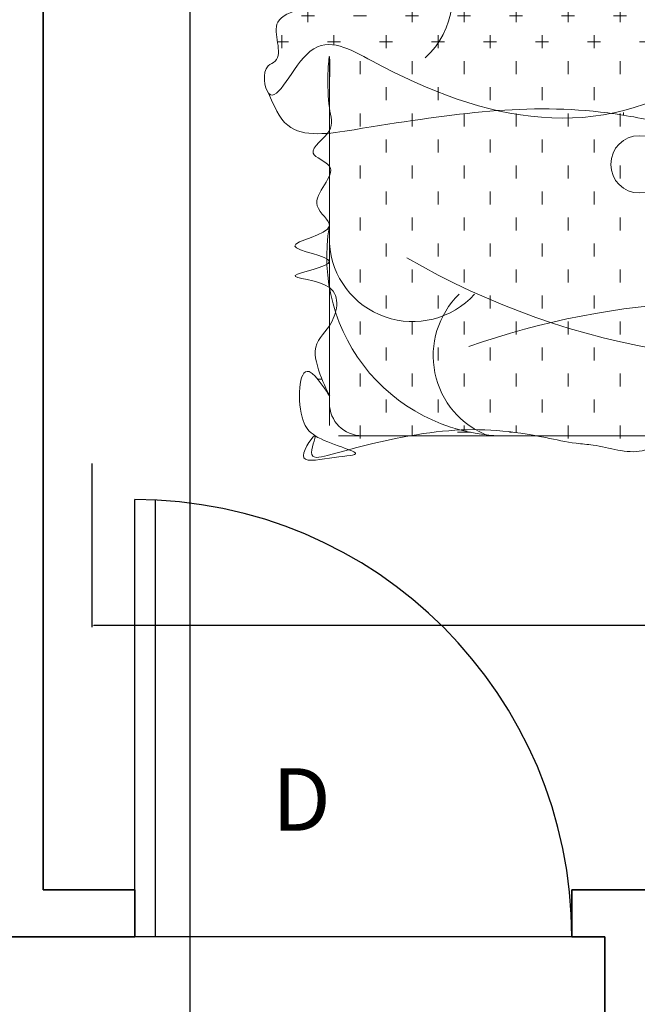
# Model space of a CAD drawing. Units: inches. Extents: x -26 to 575, y -18 to 513.
# Tile 11 of 28: x 136 to 196, y 324 to 418. Entities that reach past the tile are written whole.
import ezdxf

# ---------------------------------------------------------------- set-up
doc = ezdxf.new("R2010")
doc.units = ezdxf.units.IN
doc.header["$MEASUREMENT"] = 0
for name, color, linetype, lineweight in [('A-ANNO-DIMS', 2, 'Continuous', 18), ('A-ANNO-TEXT', 7, 'Continuous', 18), ('A-DOOR', 3, 'Continuous', 25), ('A-WALL', 7, 'Continuous', 35), ('Furniture', 8, 'Continuous', 15)]:
    doc.layers.add(name, color=color, linetype=linetype, lineweight=lineweight)
doc.styles.get("Standard").update_dxf_attribs({"font": 'arial.ttf', "height": 6})
doc.dimstyles.get("Standard").update_dxf_attribs({"dimtxt": 6, "dimasz": 0.18, "dimexe": 0.18, "dimexo": 0.0625, "dimgap": 0.09, "dimtad": 0, "dimtih": 1, "dimtoh": 1, "dimzin": 0, "dimdsep": 46, "dimlunit": 3, "dimtxsty": 'Standard', "dimcen": 0.09, "dimadec": 0, "dimazin": 0, "dimtfac": 1, "dimtofl": 0, "dimtmove": 0, "dimatfit": 3, "dimfxl": 1, "dimtolj": 1, "dimtzin": 0, "dimarcsym": 0})

# ---------------------------------------------------------------- blocks, each defined once
blk = doc.blocks.new('BED-DOUBLE-WITH-NIGHTSTANDS')
for p, q in [((1.925, 83.361), (1.925, 62.761)), ((82.669, 83.361), (82.669, 62.761)), ((21.61, 63.031), (21.61, 82.461)), ((22.828, 60.828), (22.828, 82.615)), ((81.883, 82.344), (81.883, 56.232)), ((102.354, 63.031), (102.354, 82.461)), ((10.269, 81.761), (8.938, 70.826)), ((23.226, 81.078), (0, 81.078)), ((21.24, 81.17), (81.883, 81.17)), ((103.97, 81.078), (80.744, 81.078)), ((20.889, 80.153), (2.667, 80.153)), ((2.667, 80.153), (2.667, 64.968)), ((20.889, 64.968), (20.889, 80.153)), ((82.669, 79.717), (21.062, 79.717)), ((101.633, 80.153), (83.411, 80.153)), ((83.411, 80.153), (83.411, 64.968)), ((101.633, 64.968), (101.633, 80.153)), ((92.567, 79.403), (92.567, 67.508)), ((14.667, 76.005), (4.51, 77.257)), ((25.057, 76.764), (22.828, 76.764)), ((41.168, 76.507), (40.96, 76.715)), ((41.168, 76.507), (41.434, 76.772)), ((41.169, 76.507), (41.169, 76.741)), ((56.226, 76.764), (41.357, 76.764)), ((43.997, 76.507), (43.732, 76.772)), ((43.997, 76.507), (43.997, 76.882)), ((43.997, 76.507), (44.262, 76.772)), ((46.825, 76.507), (46.56, 76.772)), ((46.825, 76.507), (47.09, 76.772)), ((46.826, 76.507), (46.826, 76.882)), ((57.003, 76.507), (56.737, 76.772)), ((57.003, 76.507), (57.003, 76.828)), ((57.003, 76.507), (57.268, 76.772)), ((81.883, 76.764), (59.394, 76.764)), ((59.831, 76.507), (59.594, 76.744)), ((59.831, 76.507), (59.831, 76.717)), ((59.831, 76.507), (60.018, 76.694)), ((8.056, 67.244), (12.026, 75.725)), ((12.026, 75.725), (14.235, 74.691)), ((11.458, 75.323), (8.122, 68.196)), ((11.769, 75.177), (11.458, 75.323)), ((25.612, 75.093), (25.347, 75.358)), ((25.612, 75.093), (25.612, 75.468)), ((25.612, 75.093), (25.877, 75.358)), ((28.44, 75.093), (28.175, 75.358)), ((28.44, 75.093), (28.706, 75.358)), ((28.441, 75.093), (28.441, 75.468)), ((31.269, 75.093), (31.004, 75.358)), ((31.269, 75.093), (31.269, 75.468)), ((31.269, 75.093), (31.534, 75.358)), ((34.097, 75.093), (33.832, 75.358)), ((34.097, 75.093), (34.362, 75.358)), ((34.098, 75.093), (34.098, 75.468)), ((36.926, 75.093), (36.661, 75.358)), ((36.926, 75.093), (36.926, 75.468)), ((36.926, 75.093), (37.191, 75.358)), ((39.754, 75.093), (39.489, 75.358)), ((39.754, 75.093), (40.019, 75.358)), ((39.755, 75.093), (39.755, 75.468)), ((42.583, 75.093), (42.317, 75.358)), ((42.583, 75.093), (42.583, 75.468)), ((42.583, 75.093), (42.848, 75.358)), ((45.411, 75.093), (45.146, 75.358)), ((45.411, 75.093), (45.411, 75.468)), ((45.411, 75.093), (45.676, 75.358)), ((48.239, 75.093), (47.974, 75.358)), ((48.239, 75.093), (48.505, 75.358)), ((48.24, 75.093), (48.24, 75.468)), ((51.068, 75.093), (50.803, 75.358)), ((51.068, 75.093), (51.068, 75.099)), ((51.068, 75.093), (51.07, 75.095)), ((53.004, 75.337), (53.025, 75.358)), ((55.588, 75.093), (55.323, 75.358)), ((55.588, 75.093), (55.854, 75.358)), ((55.589, 75.093), (55.589, 75.468)), ((58.417, 75.093), (58.152, 75.358)), ((58.417, 75.093), (58.417, 75.468)), ((58.417, 75.093), (58.682, 75.358)), ((61.245, 75.093), (60.98, 75.358)), ((61.245, 75.093), (61.51, 75.358)), ((61.246, 75.093), (61.246, 75.468)), ((64.074, 75.093), (63.809, 75.358)), ((64.074, 75.093), (64.074, 75.468)), ((64.074, 75.093), (64.339, 75.358)), ((66.902, 75.093), (66.637, 75.358)), ((66.902, 75.093), (67.167, 75.358)), ((66.903, 75.093), (66.903, 75.468)), ((69.731, 75.093), (69.465, 75.358)), ((69.731, 75.093), (69.731, 75.468)), ((69.731, 75.093), (69.996, 75.358)), ((72.559, 75.093), (72.294, 75.358)), ((72.559, 75.093), (72.559, 75.468)), ((72.559, 75.093), (72.824, 75.358)), ((75.387, 75.093), (75.122, 75.358)), ((75.387, 75.093), (75.653, 75.358)), ((75.388, 75.093), (75.388, 75.468)), ((78.216, 75.093), (77.951, 75.358)), ((78.216, 75.093), (78.216, 75.468)), ((78.216, 75.093), (78.481, 75.358)), ((14.235, 74.691), (10.265, 66.21)), ((19.14, 71.727), (13.978, 74.143)), ((27.026, 73.679), (26.761, 73.944)), ((27.026, 73.679), (27.291, 73.944)), ((27.027, 73.678), (27.027, 74.053)), ((29.855, 73.679), (29.589, 73.944)), ((29.855, 73.678), (29.855, 74.053)), ((29.855, 73.679), (30.12, 73.944)), ((32.683, 73.679), (32.418, 73.944)), ((32.683, 73.678), (32.683, 74.053)), ((32.683, 73.679), (32.948, 73.944)), ((35.512, 73.679), (35.246, 73.944)), ((35.512, 73.678), (35.512, 74.053)), ((35.512, 73.679), (35.777, 73.944)), ((38.34, 73.679), (38.075, 73.944)), ((38.34, 73.678), (38.34, 74.053)), ((38.34, 73.679), (38.605, 73.944)), ((41.168, 73.679), (40.903, 73.944)), ((41.168, 73.679), (41.434, 73.944)), ((41.169, 73.678), (41.169, 74.053)), ((43.997, 73.679), (43.732, 73.944)), ((43.997, 73.678), (43.997, 74.053)), ((43.997, 73.679), (44.262, 73.944)), ((46.825, 73.679), (46.56, 73.944)), ((46.825, 73.679), (47.09, 73.944)), ((46.826, 73.678), (46.826, 74.053)), ((49.654, 73.679), (49.388, 73.944)), ((49.654, 73.678), (49.654, 74.053)), ((49.654, 73.679), (49.919, 73.944)), ((54.174, 73.679), (53.909, 73.944)), ((54.174, 73.679), (54.439, 73.944)), ((54.175, 73.678), (54.175, 74.053)), ((57.003, 73.679), (56.737, 73.944)), ((57.003, 73.678), (57.003, 74.053)), ((57.003, 73.679), (57.268, 73.944)), ((59.831, 73.679), (59.566, 73.944)), ((59.831, 73.678), (59.831, 74.053)), ((59.831, 73.679), (60.096, 73.944)), ((62.66, 73.679), (62.394, 73.944)), ((62.66, 73.678), (62.66, 74.053)), ((62.66, 73.679), (62.925, 73.944)), ((65.488, 73.679), (65.223, 73.944)), ((65.488, 73.678), (65.488, 74.053)), ((65.488, 73.679), (65.753, 73.944)), ((68.316, 73.679), (68.051, 73.944)), ((68.316, 73.679), (68.582, 73.944)), ((68.317, 73.678), (68.317, 74.053)), ((71.145, 73.679), (70.88, 73.944)), ((71.145, 73.678), (71.145, 74.053)), ((71.145, 73.679), (71.41, 73.944)), ((73.973, 73.679), (73.708, 73.944)), ((73.973, 73.679), (74.238, 73.944)), ((73.974, 73.678), (73.974, 74.053)), ((76.802, 73.679), (76.536, 73.944)), ((76.802, 73.678), (76.802, 74.053)), ((76.802, 73.679), (77.067, 73.944)), ((79.63, 73.679), (79.365, 73.944)), ((79.63, 73.678), (79.63, 74.053)), ((79.63, 73.679), (79.895, 73.944)), ((13.242, 72.571), (11.033, 73.605)), ((14.129, 73), (11.598, 67.591)), ((17.984, 71.195), (14.129, 73)), ((98.466, 73.144), (86.668, 73.144)), ((25.612, 72.265), (25.347, 72.53)), ((25.612, 72.264), (25.612, 72.639)), ((25.612, 72.265), (25.877, 72.53)), ((28.44, 72.265), (28.175, 72.53)), ((28.44, 72.265), (28.706, 72.53)), ((28.441, 72.264), (28.441, 72.639)), ((31.269, 72.265), (31.004, 72.53)), ((31.269, 72.264), (31.269, 72.639)), ((31.269, 72.265), (31.534, 72.53)), ((34.097, 72.265), (33.832, 72.53)), ((34.097, 72.265), (34.362, 72.53)), ((34.098, 72.264), (34.098, 72.639)), ((36.926, 72.265), (36.661, 72.53)), ((36.926, 72.264), (36.926, 72.639)), ((36.926, 72.265), (37.191, 72.53)), ((39.754, 72.265), (39.489, 72.53)), ((39.754, 72.265), (40.019, 72.53)), ((39.755, 72.264), (39.755, 72.639)), ((42.583, 72.265), (42.317, 72.53)), ((42.583, 72.264), (42.583, 72.639)), ((42.583, 72.265), (42.848, 72.53)), ((45.411, 72.265), (45.146, 72.53)), ((45.411, 72.264), (45.411, 72.639)), ((45.411, 72.265), (45.676, 72.53)), ((48.239, 72.265), (47.974, 72.53)), ((48.239, 72.265), (48.505, 72.53)), ((48.24, 72.264), (48.24, 72.639)), ((55.588, 72.265), (55.323, 72.53)), ((55.588, 72.265), (55.854, 72.53)), ((55.589, 72.264), (55.589, 72.639)), ((58.417, 72.265), (58.152, 72.53)), ((58.417, 72.264), (58.417, 72.639)), ((58.417, 72.265), (58.682, 72.53)), ((61.245, 72.265), (60.98, 72.53)), ((61.245, 72.265), (61.51, 72.53)), ((61.246, 72.264), (61.246, 72.639)), ((64.074, 72.265), (63.809, 72.53)), ((64.074, 72.264), (64.074, 72.639)), ((64.074, 72.265), (64.339, 72.53)), ((66.902, 72.265), (66.637, 72.53)), ((66.902, 72.265), (67.167, 72.53)), ((66.903, 72.264), (66.903, 72.639)), ((69.731, 72.265), (69.465, 72.53)), ((69.731, 72.264), (69.731, 72.639)), ((69.731, 72.265), (69.996, 72.53)), ((72.559, 72.265), (72.294, 72.53)), ((72.559, 72.264), (72.559, 72.639)), ((72.559, 72.265), (72.824, 72.53)), ((75.387, 72.265), (75.122, 72.53)), ((75.387, 72.265), (75.653, 72.53)), ((75.388, 72.264), (75.388, 72.639)), ((78.216, 72.265), (77.951, 72.53)), ((78.216, 72.264), (78.216, 72.639)), ((78.216, 72.265), (78.481, 72.53)), ((15.452, 65.787), (17.984, 71.195)), ((15.804, 64.601), (19.14, 71.727)), ((24.198, 70.85), (23.972, 71.076)), ((24.198, 70.85), (24.198, 71.225)), ((24.198, 70.85), (24.463, 71.116)), ((27.026, 70.85), (26.761, 71.116)), ((27.026, 70.85), (27.291, 71.116)), ((27.027, 70.85), (27.027, 71.225)), ((29.855, 70.85), (29.589, 71.116)), ((29.855, 70.85), (29.855, 71.225)), ((29.855, 70.85), (30.12, 71.116)), ((32.683, 70.85), (32.418, 71.116)), ((32.683, 70.85), (32.683, 71.225)), ((32.683, 70.85), (32.948, 71.116)), ((35.512, 70.85), (35.246, 71.116)), ((35.512, 70.85), (35.512, 71.225)), ((35.512, 70.85), (35.777, 71.116)), ((38.34, 70.85), (38.075, 71.116)), ((38.34, 70.85), (38.34, 71.225)), ((38.34, 70.85), (38.605, 71.116)), ((41.168, 70.85), (40.903, 71.116)), ((41.168, 70.85), (41.434, 71.116)), ((41.169, 70.85), (41.169, 71.225)), ((43.997, 70.85), (43.732, 71.116)), ((43.997, 70.85), (43.997, 71.225)), ((43.997, 70.85), (44.262, 71.116)), ((46.825, 70.85), (46.56, 71.116)), ((46.825, 70.85), (47.09, 71.116)), ((46.826, 70.85), (46.826, 71.225)), ((49.654, 70.85), (49.388, 71.116)), ((49.654, 70.85), (49.654, 71.225)), ((49.654, 70.85), (49.919, 71.116)), ((54.174, 70.85), (53.909, 71.116)), ((54.174, 70.85), (54.439, 71.116)), ((54.175, 70.85), (54.175, 71.225)), ((57.003, 70.85), (56.737, 71.116)), ((57.003, 70.85), (57.003, 71.225)), ((57.003, 70.85), (57.268, 71.116)), ((59.831, 70.85), (59.566, 71.116)), ((59.831, 70.85), (59.831, 71.225)), ((59.831, 70.85), (60.096, 71.116)), ((62.66, 70.85), (62.394, 71.116)), ((62.66, 70.85), (62.66, 71.225)), ((62.66, 70.85), (62.925, 71.116)), ((65.488, 70.85), (65.223, 71.116)), ((65.488, 70.85), (65.488, 71.225)), ((65.488, 70.85), (65.753, 71.116)), ((68.316, 70.85), (68.051, 71.116)), ((68.316, 70.85), (68.582, 71.116)), ((68.317, 70.85), (68.317, 71.225)), ((71.145, 70.85), (70.88, 71.116)), ((71.145, 70.85), (71.145, 71.225)), ((71.145, 70.85), (71.41, 71.116)), ((73.973, 70.85), (73.708, 71.116)), ((73.973, 70.85), (74.238, 71.116)), ((73.974, 70.85), (73.974, 71.225)), ((76.802, 70.85), (76.536, 71.116)), ((76.802, 70.85), (76.802, 71.225)), ((76.802, 70.85), (77.067, 71.116)), ((79.63, 70.85), (79.365, 71.116)), ((79.63, 70.85), (79.63, 71.225)), ((79.63, 70.85), (79.895, 71.116)), ((11.136, 68.071), (8.927, 69.105)), ((25.612, 69.436), (25.347, 69.701)), ((25.612, 69.436), (25.612, 69.811)), ((25.612, 69.436), (25.877, 69.701)), ((28.44, 69.436), (28.175, 69.701)), ((28.44, 69.436), (28.706, 69.701)), ((28.441, 69.436), (28.441, 69.811)), ((31.269, 69.436), (31.004, 69.701)), ((31.269, 69.436), (31.269, 69.811)), ((31.269, 69.436), (31.534, 69.701)), ((34.097, 69.436), (33.832, 69.701)), ((34.097, 69.436), (34.362, 69.701)), ((34.098, 69.436), (34.098, 69.811)), ((36.926, 69.436), (36.661, 69.701)), ((36.926, 69.436), (36.926, 69.811)), ((36.926, 69.436), (37.191, 69.701)), ((39.754, 69.436), (39.489, 69.701)), ((39.754, 69.436), (40.019, 69.701)), ((39.755, 69.436), (39.755, 69.811)), ((42.583, 69.436), (42.317, 69.701)), ((42.583, 69.436), (42.583, 69.811)), ((42.583, 69.436), (42.848, 69.701)), ((45.411, 69.436), (45.146, 69.701)), ((45.411, 69.436), (45.411, 69.811)), ((45.411, 69.436), (45.676, 69.701)), ((48.239, 69.436), (47.974, 69.701)), ((48.239, 69.436), (48.505, 69.701)), ((48.24, 69.436), (48.24, 69.811)), ((51.052, 69.452), (50.803, 69.701)), ((53.007, 69.683), (53.025, 69.701)), ((55.588, 69.436), (55.323, 69.701)), ((55.588, 69.436), (55.854, 69.701)), ((55.589, 69.436), (55.589, 69.811)), ((58.417, 69.436), (58.152, 69.701)), ((58.417, 69.436), (58.417, 69.811)), ((58.417, 69.436), (58.682, 69.701)), ((61.245, 69.436), (60.98, 69.701)), ((61.245, 69.436), (61.51, 69.701)), ((61.246, 69.436), (61.246, 69.811)), ((64.074, 69.436), (63.809, 69.701)), ((64.074, 69.436), (64.074, 69.811)), ((64.074, 69.436), (64.339, 69.701)), ((66.902, 69.436), (66.637, 69.701)), ((66.902, 69.436), (67.167, 69.701)), ((66.903, 69.436), (66.903, 69.811)), ((69.731, 69.436), (69.465, 69.701)), ((69.731, 69.436), (69.731, 69.811)), ((69.731, 69.436), (69.996, 69.701)), ((72.559, 69.436), (72.294, 69.701)), ((72.559, 69.436), (72.559, 69.811)), ((72.559, 69.436), (72.824, 69.701)), ((75.387, 69.436), (75.122, 69.701)), ((75.387, 69.436), (75.653, 69.701)), ((75.388, 69.436), (75.388, 69.811)), ((78.216, 69.436), (77.951, 69.701)), ((78.216, 69.436), (78.216, 69.811)), ((78.216, 69.436), (78.481, 69.701)), ((8.122, 68.196), (8.434, 68.05)), ((24.198, 68.022), (23.933, 68.287)), ((24.198, 68.022), (24.198, 68.397)), ((24.198, 68.022), (24.463, 68.287)), ((27.026, 68.022), (26.761, 68.287)), ((27.026, 68.022), (27.291, 68.287)), ((27.027, 68.022), (27.027, 68.397)), ((29.855, 68.022), (29.589, 68.287)), ((29.855, 68.022), (29.855, 68.397)), ((29.855, 68.022), (30.12, 68.287)), ((32.683, 68.022), (32.418, 68.287)), ((32.683, 68.022), (32.683, 68.397)), ((32.683, 68.022), (32.948, 68.287)), ((35.512, 68.022), (35.246, 68.287)), ((35.512, 68.022), (35.512, 68.397)), ((35.512, 68.022), (35.777, 68.287)), ((38.34, 68.022), (38.075, 68.287)), ((38.34, 68.022), (38.34, 68.397)), ((38.34, 68.022), (38.605, 68.287)), ((41.168, 68.022), (40.903, 68.287)), ((41.168, 68.022), (41.434, 68.287)), ((41.169, 68.022), (41.169, 68.397)), ((43.997, 68.022), (43.732, 68.287)), ((43.997, 68.022), (43.997, 68.397)), ((43.997, 68.022), (44.262, 68.287)), ((46.825, 68.022), (46.56, 68.287)), ((46.825, 68.022), (47.09, 68.287)), ((46.826, 68.022), (46.826, 68.397)), ((49.654, 68.022), (49.388, 68.287)), ((49.654, 68.022), (49.654, 68.397)), ((49.654, 68.022), (49.919, 68.287)), ((54.174, 68.022), (53.909, 68.287)), ((54.174, 68.022), (54.439, 68.287)), ((54.175, 68.022), (54.175, 68.397)), ((57.003, 68.022), (56.737, 68.287)), ((57.003, 68.022), (57.003, 68.397)), ((57.003, 68.022), (57.268, 68.287)), ((59.831, 68.022), (59.566, 68.287)), ((59.831, 68.022), (59.831, 68.397)), ((59.831, 68.022), (60.096, 68.287)), ((62.66, 68.022), (62.394, 68.287)), ((62.66, 68.022), (62.66, 68.397)), ((62.66, 68.022), (62.925, 68.287)), ((65.488, 68.022), (65.223, 68.287)), ((65.488, 68.022), (65.488, 68.397)), ((65.488, 68.022), (65.753, 68.287)), ((68.316, 68.022), (68.051, 68.287)), ((68.316, 68.022), (68.582, 68.287)), ((68.317, 68.022), (68.317, 68.397)), ((71.145, 68.022), (70.88, 68.287)), ((71.145, 68.022), (71.145, 68.397)), ((71.145, 68.022), (71.41, 68.287)), ((73.973, 68.022), (73.708, 68.287)), ((73.973, 68.022), (74.238, 68.287)), ((73.974, 68.022), (73.974, 68.397)), ((76.802, 68.022), (76.536, 68.287)), ((76.802, 68.022), (76.802, 68.397)), ((76.802, 68.022), (77.067, 68.287)), ((79.63, 68.022), (79.365, 68.287)), ((79.63, 68.022), (79.63, 68.397)), ((79.63, 68.022), (79.895, 68.287)), ((10.265, 66.21), (8.056, 67.244)), ((11.598, 67.591), (15.452, 65.787)), ((10.642, 67.017), (15.804, 64.601)), ((25.612, 66.608), (25.347, 66.873)), ((25.612, 66.607), (25.612, 66.982)), ((25.612, 66.608), (25.877, 66.873)), ((28.44, 66.608), (28.175, 66.873)), ((28.44, 66.608), (28.706, 66.873)), ((28.441, 66.607), (28.441, 66.982)), ((31.269, 66.608), (31.004, 66.873)), ((31.269, 66.607), (31.269, 66.982)), ((31.269, 66.608), (31.534, 66.873)), ((34.097, 66.608), (33.832, 66.873)), ((34.097, 66.608), (34.362, 66.873)), ((34.098, 66.607), (34.098, 66.982)), ((36.926, 66.608), (36.661, 66.873)), ((36.926, 66.607), (36.926, 66.982)), ((36.926, 66.608), (37.191, 66.873)), ((39.754, 66.608), (39.489, 66.873)), ((39.754, 66.608), (40.019, 66.873)), ((39.755, 66.607), (39.755, 66.982)), ((42.583, 66.608), (42.317, 66.873)), ((42.583, 66.607), (42.583, 66.982)), ((42.583, 66.608), (42.848, 66.873)), ((45.411, 66.608), (45.146, 66.873)), ((45.411, 66.607), (45.411, 66.982)), ((45.411, 66.608), (45.676, 66.873)), ((48.239, 66.608), (47.974, 66.873)), ((48.239, 66.608), (48.505, 66.873)), ((48.24, 66.607), (48.24, 66.982)), ((51.068, 66.608), (50.803, 66.873)), ((51.068, 66.607), (51.068, 66.982)), ((51.068, 66.608), (51.333, 66.873)), ((52.76, 66.608), (52.495, 66.873)), ((52.76, 66.607), (52.76, 66.982)), ((52.76, 66.608), (53.025, 66.873)), ((55.588, 66.608), (55.323, 66.873)), ((55.588, 66.608), (55.854, 66.873)), ((55.589, 66.607), (55.589, 66.982)), ((58.417, 66.608), (58.152, 66.873)), ((58.417, 66.607), (58.417, 66.982)), ((58.417, 66.608), (58.682, 66.873)), ((61.245, 66.608), (60.98, 66.873)), ((61.245, 66.608), (61.51, 66.873)), ((61.246, 66.607), (61.246, 66.982)), ((64.074, 66.608), (63.809, 66.873)), ((64.074, 66.607), (64.074, 66.982)), ((64.074, 66.608), (64.339, 66.873)), ((66.902, 66.608), (66.637, 66.873)), ((66.902, 66.608), (67.167, 66.873)), ((66.903, 66.607), (66.903, 66.982)), ((69.731, 66.608), (69.465, 66.873)), ((69.731, 66.607), (69.731, 66.982)), ((69.731, 66.608), (69.996, 66.873)), ((72.559, 66.608), (72.294, 66.873)), ((72.559, 66.607), (72.559, 66.982)), ((72.559, 66.608), (72.824, 66.873)), ((75.387, 66.608), (75.122, 66.873)), ((75.387, 66.608), (75.653, 66.873)), ((75.388, 66.607), (75.388, 66.982)), ((78.216, 66.608), (77.951, 66.873)), ((78.216, 66.607), (78.216, 66.982)), ((78.216, 66.608), (78.481, 66.873)), ((81.044, 66.608), (80.779, 66.873)), ((81.044, 66.608), (81.253, 66.817)), ((81.045, 66.607), (81.045, 66.982)), ((24.198, 65.385), (24.198, 65.568)), ((24.295, 65.291), (24.463, 65.459)), ((27.026, 65.194), (26.761, 65.459)), ((27.026, 65.194), (27.291, 65.459)), ((27.027, 65.193), (27.027, 65.568)), ((29.855, 65.194), (29.589, 65.459)), ((29.855, 65.193), (29.855, 65.568)), ((29.855, 65.194), (30.12, 65.459)), ((32.683, 65.194), (32.418, 65.459)), ((32.683, 65.193), (32.683, 65.568)), ((32.683, 65.194), (32.948, 65.459)), ((35.335, 65.37), (35.246, 65.459)), ((35.512, 65.394), (35.512, 65.568)), ((35.743, 65.425), (35.777, 65.459)), ((46.774, 65.245), (46.56, 65.459)), ((46.826, 65.232), (46.826, 65.568)), ((46.856, 65.224), (47.09, 65.459)), ((49.654, 65.194), (49.388, 65.459)), ((49.654, 65.193), (49.654, 65.568)), ((49.654, 65.194), (49.919, 65.459)), ((54.174, 65.194), (53.909, 65.459)), ((54.174, 65.194), (54.439, 65.459)), ((54.175, 65.193), (54.175, 65.568)), ((57.003, 65.194), (56.737, 65.459)), ((57.003, 65.193), (57.003, 65.568)), ((57.003, 65.194), (57.268, 65.459)), ((59.831, 65.194), (59.566, 65.459)), ((59.831, 65.193), (59.831, 65.568)), ((59.831, 65.194), (60.096, 65.459)), ((62.66, 65.525), (62.66, 65.568)), ((65.488, 65.481), (65.488, 65.568)), ((65.74, 65.446), (65.753, 65.459)), ((68.316, 65.194), (68.051, 65.459)), ((68.316, 65.194), (68.582, 65.459)), ((68.317, 65.193), (68.317, 65.568)), ((71.145, 65.194), (70.88, 65.459)), ((71.145, 65.193), (71.145, 65.568)), ((71.145, 65.194), (71.41, 65.459)), ((73.973, 65.194), (73.708, 65.459)), ((73.973, 65.194), (74.238, 65.459)), ((73.974, 65.193), (73.974, 65.568)), ((76.802, 65.194), (76.536, 65.459)), ((76.802, 65.193), (76.802, 65.568)), ((76.802, 65.194), (77.067, 65.459)), ((79.63, 65.194), (79.365, 65.459)), ((79.63, 65.193), (79.63, 65.568)), ((79.63, 65.194), (79.895, 65.459)), ((82.154, 61.735), (82.154, 65.422)), ((2.667, 64.968), (20.889, 64.968)), ((83.411, 64.968), (101.633, 64.968)), ((0.451, 64.149), (23.136, 64.149)), ((55.589, 64.121), (55.589, 64.154)), ((81.194, 64.149), (103.88, 64.149)), ((78.267, 59.667), (78.267, 60.149)), ((20.767, 58.212), (20.767, 58.417)), ((21.392, 57.792), (21.312, 57.792)), ((26.392, 57.792), (25.142, 57.792)), ((25.767, 57.167), (25.767, 58.417)), ((31.392, 57.792), (30.142, 57.792)), ((30.767, 57.167), (30.767, 58.417)), ((36.392, 57.792), (35.142, 57.792)), ((35.767, 57.167), (35.767, 58.407)), ((41.392, 57.792), (40.142, 57.792)), ((40.767, 57.167), (40.767, 57.965)), ((60.767, 57.167), (60.767, 57.735)), ((66.392, 57.792), (65.142, 57.792)), ((65.767, 57.167), (65.767, 58.213)), ((71.392, 57.792), (70.142, 57.792)), ((70.767, 57.167), (70.767, 58.417)), ((76.392, 57.792), (75.142, 57.792)), ((75.767, 57.167), (75.767, 58.417)), ((81.392, 57.792), (80.142, 57.792)), ((80.767, 57.167), (80.767, 58.417)), ((45.767, 57.167), (45.767, 57.639)), ((50.767, 57.167), (50.767, 57.462)), ((55.767, 57.167), (55.767, 57.483)), ((28.267, 54.667), (28.267, 55.917)), ((33.267, 54.667), (33.267, 55.917)), ((38.267, 54.667), (38.267, 55.917)), ((43.267, 54.667), (43.267, 55.917)), ((48.267, 54.667), (48.267, 55.917)), ((53.267, 54.667), (53.267, 55.917)), ((58.267, 54.667), (58.267, 55.917)), ((63.267, 54.667), (63.267, 55.917)), ((68.267, 54.667), (68.267, 55.917)), ((73.267, 54.667), (73.267, 55.917)), ((78.267, 54.667), (78.267, 55.917)), ((83.267, 54.667), (83.267, 55.917)), ((23.273, 54.636), (23.273, 55.755)), ((28.892, 55.292), (27.642, 55.292)), ((33.892, 55.292), (32.642, 55.292)), ((38.892, 55.292), (37.642, 55.292)), ((43.892, 55.292), (42.642, 55.292)), ((48.892, 55.292), (47.642, 55.292)), ((53.892, 55.292), (52.642, 55.292)), ((58.892, 55.292), (57.642, 55.292)), ((63.892, 55.292), (62.642, 55.292)), ((68.892, 55.292), (67.642, 55.292)), ((73.892, 55.292), (72.642, 55.292)), ((78.892, 55.292), (77.642, 55.292)), ((83.892, 55.292), (82.642, 55.292)), ((30.767, 52.167), (30.767, 53.417)), ((35.767, 52.167), (35.767, 53.417)), ((40.767, 52.167), (40.767, 53.417)), ((45.767, 52.167), (45.767, 53.417)), ((50.767, 52.167), (50.767, 53.417)), ((55.767, 52.167), (55.767, 53.417)), ((60.767, 52.167), (60.767, 53.417)), ((65.767, 52.167), (65.767, 53.417)), ((70.767, 52.167), (70.767, 53.417)), ((75.767, 52.167), (75.767, 53.417)), ((80.767, 52.167), (80.767, 53.417)), ((26.392, 52.792), (25.619, 52.792)), ((31.392, 52.792), (30.142, 52.792)), ((36.392, 52.792), (35.142, 52.792)), ((41.392, 52.792), (40.142, 52.792)), ((46.392, 52.792), (45.142, 52.792)), ((51.392, 52.792), (50.142, 52.792)), ((56.392, 52.792), (55.142, 52.792)), ((61.392, 52.792), (60.142, 52.792)), ((66.392, 52.792), (65.142, 52.792)), ((71.392, 52.792), (70.142, 52.792)), ((76.392, 52.792), (75.142, 52.792)), ((81.392, 52.792), (80.142, 52.792)), ((23.892, 50.292), (22.642, 50.292)), ((23.267, 49.667), (23.267, 50.917)), ((28.892, 50.292), (27.642, 50.292)), ((28.267, 49.667), (28.267, 50.917)), ((33.892, 50.292), (32.642, 50.292)), ((33.267, 49.667), (33.267, 50.917)), ((38.892, 50.292), (37.642, 50.292)), ((38.267, 49.667), (38.267, 50.917)), ((43.892, 50.292), (42.642, 50.292)), ((43.267, 49.667), (43.267, 50.917)), ((48.892, 50.292), (47.642, 50.292)), ((48.267, 49.667), (48.267, 50.917)), ((53.892, 50.292), (52.642, 50.292)), ((53.267, 49.667), (53.267, 50.917)), ((58.892, 50.292), (57.642, 50.292)), ((58.267, 49.667), (58.267, 50.917)), ((63.892, 50.292), (62.642, 50.292)), ((63.267, 49.667), (63.267, 50.917)), ((68.892, 50.292), (67.642, 50.292)), ((68.267, 49.667), (68.267, 50.917)), ((73.892, 50.292), (72.642, 50.292)), ((73.267, 49.667), (73.267, 50.917)), ((78.892, 50.292), (77.642, 50.292)), ((78.267, 49.667), (78.267, 50.917)), ((83.892, 50.292), (82.642, 50.292)), ((83.267, 49.667), (83.267, 50.917)), ((20.767, 47.167), (20.767, 48.417)), ((30.767, 47.167), (30.767, 48.417)), ((35.767, 47.167), (35.767, 48.417)), ((40.767, 47.167), (40.767, 48.417)), ((45.767, 47.167), (45.767, 48.417)), ((50.767, 47.167), (50.767, 48.417)), ((55.767, 47.167), (55.767, 48.417)), ((65.767, 47.167), (65.767, 48.417)), ((70.767, 47.167), (70.767, 48.417)), ((75.767, 47.167), (75.767, 48.417)), ((80.767, 47.167), (80.767, 48.417)), ((21.392, 47.792), (20.412, 47.792)), ((26.392, 47.792), (25.142, 47.792)), ((31.392, 47.792), (30.142, 47.792)), ((36.392, 47.792), (35.142, 47.792)), ((41.392, 47.792), (40.142, 47.792)), ((46.392, 47.792), (45.142, 47.792)), ((51.392, 47.792), (50.142, 47.792)), ((56.392, 47.792), (55.142, 47.792)), ((66.392, 47.792), (65.142, 47.792)), ((71.392, 47.792), (70.142, 47.792)), ((76.392, 47.792), (75.142, 47.792)), ((81.392, 47.792), (80.142, 47.792)), ((23.267, 44.667), (23.267, 45.917)), ((28.267, 44.667), (28.267, 45.917)), ((33.267, 44.667), (33.267, 45.917)), ((38.267, 44.667), (38.267, 45.917)), ((43.267, 44.667), (43.267, 45.917)), ((48.267, 44.667), (48.267, 45.917)), ((53.267, 44.667), (53.267, 45.917)), ((63.267, 44.667), (63.267, 45.917)), ((68.267, 44.667), (68.267, 45.917)), ((73.267, 44.667), (73.267, 45.917)), ((78.267, 44.667), (78.267, 45.917)), ((83.267, 44.667), (83.267, 45.917)), ((23.892, 45.292), (22.642, 45.292)), ((28.892, 45.292), (27.642, 45.292)), ((33.892, 45.292), (32.642, 45.292)), ((38.892, 45.292), (37.642, 45.292)), ((43.892, 45.292), (42.642, 45.292)), ((48.892, 45.292), (47.642, 45.292)), ((53.892, 45.292), (52.642, 45.292)), ((58.892, 45.292), (57.642, 45.292)), ((63.892, 45.292), (62.642, 45.292)), ((68.892, 45.292), (67.642, 45.292)), ((73.892, 45.292), (72.642, 45.292)), ((78.892, 45.292), (77.642, 45.292)), ((83.892, 45.292), (82.642, 45.292)), ((21.392, 42.792), (20.142, 42.792)), ((20.767, 42.167), (20.767, 43.417)), ((26.392, 42.792), (25.142, 42.792)), ((31.392, 42.792), (30.142, 42.792)), ((30.767, 42.167), (30.767, 43.417)), ((36.392, 42.792), (35.142, 42.792)), ((35.767, 42.167), (35.767, 43.417)), ((41.392, 42.792), (40.142, 42.792)), ((40.767, 42.167), (40.767, 43.417)), ((46.392, 42.792), (45.142, 42.792)), ((45.767, 42.167), (45.767, 43.417)), ((51.392, 42.792), (50.142, 42.792)), ((50.767, 42.167), (50.767, 43.417)), ((56.392, 42.792), (55.142, 42.792)), ((55.767, 42.167), (55.767, 43.417)), ((61.392, 42.792), (60.142, 42.792)), ((66.089, 42.792), (65.142, 42.792)), ((65.767, 42.167), (65.767, 43.417)), ((70.767, 42.167), (70.767, 43.417)), ((75.767, 42.167), (75.767, 43.417)), ((76.392, 42.792), (76.07, 42.792)), ((81.392, 42.792), (80.142, 42.792)), ((80.767, 42.167), (80.767, 43.417)), ((86.392, 42.792), (85.142, 42.792)), ((85.767, 42.167), (85.767, 43.417)), ((72.149, 42.386), (71.41, 42.386)), ((71.779, 42.017), (71.779, 42.495)), ((81.883, 42.36), (81.883, 0)), ((18.267, 39.667), (18.267, 40.917)), ((23.267, 39.991), (23.267, 40.917)), ((28.267, 39.667), (28.267, 40.917)), ((33.267, 39.667), (33.267, 40.917)), ((38.267, 39.667), (38.267, 40.917)), ((43.267, 39.667), (43.267, 40.917)), ((48.267, 39.667), (48.267, 40.917)), ((53.267, 39.667), (53.267, 40.917)), ((63.267, 39.667), (63.267, 40.917)), ((67.35, 40.541), (67.35, 40.835)), ((67.719, 40.91), (67.48, 40.91)), ((68.267, 39.667), (68.267, 40.917)), ((70.672, 40.91), (69.934, 40.91)), ((70.303, 40.541), (70.303, 41.279)), ((73.625, 40.91), (72.887, 40.91)), ((73.256, 40.541), (73.256, 41.279)), ((73.267, 39.667), (73.267, 40.917)), ((76.578, 40.91), (75.839, 40.91)), ((76.209, 40.541), (76.209, 41.133)), ((78.267, 39.667), (78.267, 40.917)), ((83.267, 39.667), (83.267, 40.917)), ((18.892, 40.292), (17.831, 40.292)), ((23.892, 40.292), (22.642, 40.292)), ((28.892, 40.292), (27.642, 40.292)), ((33.892, 40.292), (32.642, 40.292)), ((38.892, 40.292), (37.642, 40.292)), ((43.892, 40.292), (42.642, 40.292)), ((48.892, 40.292), (47.642, 40.292)), ((53.892, 40.292), (52.642, 40.292)), ((58.892, 40.292), (57.642, 40.292)), ((62.901, 40.292), (62.642, 40.292)), ((65.874, 39.064), (65.874, 39.802)), ((68.827, 39.064), (68.827, 39.802)), ((71.779, 39.064), (71.779, 39.802)), ((74.732, 39.064), (74.732, 39.802)), ((77.685, 39.064), (77.685, 39.802)), ((83.892, 40.292), (82.642, 40.292)), ((22.828, 3.418), (22.828, 38.865)), ((66.243, 39.433), (65.505, 39.433)), ((69.196, 39.433), (68.458, 39.433)), ((72.149, 39.433), (71.41, 39.433)), ((75.101, 39.433), (74.363, 39.433)), ((78.054, 39.433), (77.316, 39.433)), ((25.767, 37.167), (25.767, 38.417)), ((30.767, 37.167), (30.767, 38.417)), ((35.767, 37.167), (35.767, 38.417)), ((40.767, 37.167), (40.767, 38.417)), ((45.767, 37.167), (45.767, 38.417)), ((50.767, 37.167), (50.767, 38.417)), ((55.767, 37.167), (55.767, 38.417)), ((60.767, 37.167), (60.767, 38.417)), ((64.767, 37.957), (64.028, 37.957)), ((64.398, 37.588), (64.398, 38.326)), ((65.767, 37.167), (65.767, 38.417)), ((67.719, 37.957), (66.981, 37.957)), ((67.35, 37.588), (67.35, 38.326)), ((70.672, 37.957), (69.934, 37.957)), ((70.303, 37.588), (70.303, 38.326)), ((70.767, 37.167), (70.767, 38.417)), ((73.625, 37.957), (72.887, 37.957)), ((73.256, 37.588), (73.256, 38.326)), ((75.767, 37.167), (75.767, 38.417)), ((76.451, 37.957), (75.839, 37.957)), ((76.209, 37.798), (76.209, 38.326)), ((80.767, 37.167), (80.767, 38.417)), ((61.392, 37.792), (60.142, 37.792)), ((66.392, 37.792), (65.142, 37.792)), ((71.392, 37.792), (70.142, 37.792)), ((76.392, 37.792), (75.142, 37.792)), ((81.392, 37.792), (80.142, 37.792)), ((59.968, 36.111), (59.968, 36.158)), ((63.29, 36.481), (62.552, 36.481)), ((62.921, 36.111), (62.921, 36.85)), ((66.243, 36.481), (65.505, 36.481)), ((65.874, 36.111), (65.874, 36.85)), ((69.196, 36.481), (68.458, 36.481)), ((68.827, 36.111), (68.827, 36.85)), ((72.149, 36.481), (71.41, 36.481)), ((71.779, 36.111), (71.779, 36.85)), ((74.53, 36.481), (74.363, 36.481)), ((74.732, 36.661), (74.732, 36.85)), ((17.658, 35.292), (17.642, 35.292)), ((28.267, 34.667), (28.267, 35.917)), ((33.267, 34.667), (33.267, 35.917)), ((38.267, 34.667), (38.267, 35.917)), ((43.267, 34.667), (43.267, 35.917)), ((48.267, 34.667), (48.267, 35.917)), ((53.267, 34.667), (53.267, 35.917)), ((58.892, 35.292), (57.642, 35.292)), ((58.267, 34.667), (58.267, 35.917)), ((58.492, 34.635), (58.492, 35.373)), ((61.445, 34.635), (61.445, 35.373)), ((63.892, 35.292), (62.642, 35.292)), ((63.267, 34.667), (63.267, 35.917)), ((64.398, 34.635), (64.398, 35.373)), ((67.35, 34.635), (67.35, 35.373)), ((68.892, 35.292), (67.642, 35.292)), ((68.267, 34.667), (68.267, 35.917)), ((70.303, 34.635), (70.303, 35.373)), ((73.892, 35.292), (72.642, 35.292)), ((73.256, 35.252), (73.256, 35.373)), ((73.267, 34.667), (73.267, 35.917)), ((78.892, 35.292), (77.642, 35.292)), ((78.267, 34.667), (78.267, 35.917)), ((58.861, 35.004), (58.123, 35.004)), ((61.814, 35.004), (61.076, 35.004)), ((64.767, 35.004), (64.028, 35.004)), ((67.719, 35.004), (66.981, 35.004)), ((70.672, 35.004), (69.934, 35.004)), ((73.008, 35.004), (72.887, 35.004)), ((25.767, 32.167), (25.767, 33.417)), ((30.767, 32.167), (30.767, 33.417)), ((35.767, 32.167), (35.767, 33.417)), ((40.767, 32.167), (40.767, 33.417)), ((45.767, 32.167), (45.767, 33.417)), ((50.767, 32.167), (50.767, 33.417)), ((51.11, 33.245), (51.11, 33.484)), ((54.432, 33.528), (53.694, 33.528)), ((54.063, 33.159), (54.063, 33.897)), ((55.767, 32.167), (55.767, 33.417)), ((57.385, 33.528), (56.647, 33.528)), ((57.016, 33.159), (57.016, 33.897)), ((60.338, 33.528), (59.599, 33.528)), ((59.968, 33.159), (59.968, 33.897)), ((60.767, 32.167), (60.767, 33.417)), ((63.29, 33.528), (62.552, 33.528)), ((62.921, 33.159), (62.921, 33.897)), ((66.243, 33.528), (65.505, 33.528)), ((65.767, 32.167), (65.767, 33.417)), ((65.874, 33.159), (65.874, 33.897)), ((69.196, 33.528), (68.458, 33.528)), ((68.827, 33.159), (68.827, 33.897)), ((70.767, 32.167), (70.767, 33.417)), ((71.469, 33.528), (71.41, 33.528)), ((71.779, 33.808), (71.779, 33.897)), ((75.767, 32.167), (75.767, 33.417)), ((80.767, 32.167), (80.767, 33.417)), ((55.539, 32.371), (55.539, 32.421)), ((58.492, 31.744), (58.492, 32.421)), ((61.445, 31.682), (61.445, 32.421)), ((64.398, 31.682), (64.398, 32.421)), ((67.35, 31.682), (67.35, 32.421)), ((58.861, 32.051), (58.123, 32.051)), ((61.814, 32.051), (61.076, 32.051)), ((64.767, 32.051), (64.028, 32.051)), ((67.719, 32.051), (66.981, 32.051)), ((28.267, 29.667), (28.267, 30.917)), ((33.267, 29.667), (33.267, 30.917)), ((38.267, 29.667), (38.267, 30.917)), ((43.267, 29.667), (43.267, 30.917)), ((48.267, 29.667), (48.267, 30.917)), ((53.267, 29.667), (53.267, 30.917)), ((58.267, 29.667), (58.267, 30.917)), ((63.267, 29.667), (63.267, 30.917)), ((68.267, 29.667), (68.267, 30.917)), ((73.267, 29.667), (73.267, 30.917)), ((78.267, 29.667), (78.267, 30.917)), ((83.267, 29.667), (83.267, 30.107)), ((25.767, 27.167), (25.767, 28.417)), ((30.767, 27.167), (30.767, 28.417)), ((35.767, 27.167), (35.767, 28.417)), ((40.767, 27.167), (40.767, 28.417)), ((45.767, 27.167), (45.767, 28.417)), ((50.767, 27.167), (50.767, 28.417)), ((55.767, 27.167), (55.767, 28.417)), ((60.767, 27.167), (60.767, 28.417)), ((65.767, 27.167), (65.767, 28.417)), ((70.767, 27.167), (70.767, 28.417)), ((75.767, 27.167), (75.767, 28.417)), ((80.767, 27.167), (80.767, 28.417)), ((28.267, 24.667), (28.267, 25.917)), ((33.267, 24.667), (33.267, 25.917)), ((38.267, 24.667), (38.267, 25.917)), ((43.267, 24.667), (43.267, 25.917)), ((48.267, 24.667), (48.267, 25.917)), ((53.267, 24.667), (53.267, 25.917)), ((58.267, 24.667), (58.267, 25.917)), ((63.267, 24.667), (63.267, 25.917)), ((68.267, 24.667), (68.267, 25.917)), ((73.267, 24.667), (73.267, 25.917)), ((78.267, 24.667), (78.267, 25.917)), ((25.767, 22.167), (25.767, 23.417)), ((30.767, 22.167), (30.767, 23.417)), ((35.767, 22.167), (35.767, 23.417)), ((40.767, 22.167), (40.767, 23.417)), ((45.767, 22.167), (45.767, 23.417)), ((50.767, 22.167), (50.767, 23.417)), ((55.767, 22.167), (55.767, 23.417)), ((60.767, 22.167), (60.767, 23.417)), ((65.767, 22.167), (65.767, 23.417)), ((70.767, 22.167), (70.767, 23.417)), ((75.767, 22.167), (75.767, 23.417)), ((80.767, 22.167), (80.767, 23.417)), ((28.267, 19.667), (28.267, 20.917)), ((33.267, 19.667), (33.267, 20.917)), ((38.267, 19.667), (38.267, 20.917)), ((43.267, 19.667), (43.267, 20.917)), ((48.267, 19.667), (48.267, 20.917)), ((53.267, 19.667), (53.267, 20.917)), ((58.267, 19.667), (58.267, 20.917)), ((63.267, 19.667), (63.267, 20.917)), ((68.267, 19.667), (68.267, 20.917)), ((73.267, 19.667), (73.267, 20.917)), ((78.267, 19.667), (78.267, 20.917)), ((25.767, 17.168), (25.767, 18.417)), ((30.767, 17.168), (30.767, 18.417)), ((35.767, 17.168), (35.767, 18.417)), ((40.767, 17.168), (40.767, 18.417)), ((45.767, 17.168), (45.767, 18.417)), ((50.767, 17.168), (50.767, 18.417)), ((55.767, 17.168), (55.767, 18.417)), ((60.767, 17.168), (60.767, 18.417)), ((65.767, 17.168), (65.767, 18.417)), ((70.767, 17.168), (70.767, 18.417)), ((75.767, 17.168), (75.767, 18.417)), ((80.767, 17.168), (80.767, 18.417)), ((28.267, 14.668), (28.267, 15.918)), ((33.267, 14.668), (33.267, 15.918)), ((38.267, 14.668), (38.267, 15.918)), ((43.267, 14.668), (43.267, 15.918)), ((48.267, 14.668), (48.267, 15.918)), ((53.267, 14.668), (53.267, 15.918)), ((58.267, 14.668), (58.267, 15.918)), ((63.267, 14.668), (63.267, 15.918)), ((68.267, 14.668), (68.267, 15.918)), ((73.267, 14.668), (73.267, 15.918)), ((78.267, 14.668), (78.267, 15.918)), ((83.267, 15.255), (83.267, 15.918)), ((25.767, 12.168), (25.767, 13.418)), ((30.767, 12.168), (30.767, 13.418)), ((35.767, 12.168), (35.767, 13.418)), ((40.767, 12.168), (40.767, 13.418)), ((45.767, 12.168), (45.767, 13.418)), ((50.767, 12.168), (50.767, 13.418)), ((55.767, 12.168), (55.767, 13.418)), ((60.767, 12.168), (60.767, 13.418)), ((65.767, 12.168), (65.767, 13.418)), ((70.767, 12.168), (70.767, 13.418)), ((75.767, 12.168), (75.767, 13.418)), ((80.767, 12.168), (80.767, 13.418)), ((28.267, 9.668), (28.267, 10.918)), ((33.267, 9.668), (33.267, 10.918)), ((38.267, 9.668), (38.267, 10.918)), ((43.267, 9.668), (43.267, 10.918)), ((48.267, 9.668), (48.267, 10.918)), ((53.267, 9.668), (53.267, 10.918)), ((58.267, 9.668), (58.267, 10.918)), ((63.267, 9.668), (63.267, 10.918)), ((68.267, 9.668), (68.267, 10.918)), ((73.267, 9.668), (73.267, 10.918)), ((78.267, 9.668), (78.267, 10.918)), ((83.267, 9.668), (83.267, 10.196)), ((22.115, 7.867), (21.706, 7.867)), ((25.767, 7.168), (25.767, 8.418)), ((30.767, 7.168), (30.767, 8.418)), ((35.767, 7.168), (35.767, 8.418)), ((40.767, 7.168), (40.767, 8.418)), ((45.767, 7.168), (45.767, 8.418)), ((50.767, 7.168), (50.767, 8.418)), ((55.767, 7.168), (55.767, 8.418)), ((60.767, 7.168), (60.767, 8.418)), ((65.767, 7.168), (65.767, 8.418)), ((70.767, 7.168), (70.767, 8.418)), ((75.767, 7.168), (75.767, 8.418)), ((80.767, 7.168), (80.767, 8.418)), ((28.267, 4.668), (28.267, 5.918)), ((33.267, 4.668), (33.267, 5.918)), ((38.267, 4.668), (38.267, 5.918)), ((43.267, 4.668), (43.267, 5.918)), ((48.267, 4.668), (48.267, 5.918)), ((53.267, 4.668), (53.267, 5.918)), ((58.267, 4.668), (58.267, 5.918)), ((63.267, 4.668), (63.267, 5.918)), ((68.267, 4.668), (68.267, 5.918)), ((73.267, 4.668), (73.267, 5.918)), ((78.267, 4.668), (78.267, 5.918)), ((25.767, 2.168), (25.767, 3.418)), ((30.767, 2.465), (30.767, 3.418)), ((35.767, 3.004), (35.767, 3.418)), ((40.767, 2.745), (40.767, 3.418)), ((45.767, 2.168), (45.767, 3.418)), ((50.767, 2.168), (50.767, 3.418)), ((55.767, 2.168), (55.767, 3.418)), ((60.767, 2.168), (60.767, 3.418)), ((65.767, 2.168), (65.767, 3.418)), ((70.767, 2.168), (70.767, 3.418)), ((75.767, 2.413), (75.767, 3.418)), ((80.767, 2.168), (80.767, 3.418)), ((85.58, 2.43), (23.697, 2.43)), ((36.392, 2.793), (35.142, 2.793)), ((40.395, 2.793), (40.142, 2.793))]:
    blk.add_line(p, q)
for centre, radius in [((9.65, 76.677), 4.065), ((9.65, 76.677), 3.73), ((9.65, 76.677), 1.87), ((9.65, 76.677), 1.702), ((92.824, 73.144), 3.847), ((92.824, 73.144), 2.272), ((60.492, 47.373), 2.359), ((52.627, 28.516), 2.753)]:
    blk.add_circle(centre, radius)
for centre, radius, start, end in [((40.615, 70.411), 11.457, 327.75554, 34.13971), ((18.641, 72.674), 7.534, 354.32477, 27.77276), ((41.09, 50.385), 26.004, 95.02643, 117.32994), ((64.238, 66.161), 9.788, 78.78839, 122.5362), ((83.338, 72.35), 4.658, 124.73446, 186.55264), ((44.415, 57.102), 10.589, 48.87132, 93.34478), ((76.199, 84.696), 20.356, 248.18569, 275.91055), ((27.055, 44.467), 7.557, 311.04012, 36.13845), ((86.259, 43.416), 4.944, 128.83543, 178.00379), ((39.784, 19.641), 17.214, 170.06779, 270.93205), ((30.825, 21.414), 8.013, 183.53609, 317.84857), ((66.971, 82.605), 72.965, 239.8126, 282.54723), ((41.047, 10.13), 8.244, 134.23532, 249.05847), ((61.483, -60.526), 75.853, 75.71433, 109.44594), ((25.975, 5.579), 3.15, 180, 270), ((78.733, 5.579), 3.15, 270, 0)]:
    blk.add_arc(centre, radius, start, end)
for points, knots in [([(24.713, 64.661), (26.06, 64.632), (33.003, 64.48), (41.955, 67.204), (49.025, 64.485), (52.786, 64.865), (50.633, 69.88), (50.431, 72.758), (51.756, 76.03), (43.447, 78.051), (36.588, 75.072), (28.311, 76.389), (25.374, 76.358), (24.839, 76.353)], [0, 0, 0, 0, 4.049674, 20.880819, 25.932041, 26.821979, 31.217024, 36.043065, 37.533831, 40.150607, 55.448466, 62.672935, 64.278467, 64.278467, 64.278467, 64.278467]), ([(81.301, 78.042), (80.682, 75.308), (79.671, 70.849), (81.18, 67.616), (83.379, 62.518), (82.094, 64.567), (81.589, 64.661)], [0, 0, 0, 0, 7.603099, 12.404488, 14.892294, 16.432626, 16.432626, 16.432626, 16.432626]), ([(25.073, 76.86), (24.732, 74.842), (24.154, 71.41), (22.763, 66.411), (24.846, 64.896), (25.601, 63.748), (26.066, 63.834)], [0, 0, 0, 0, 6.47304, 11.006869, 12.799679, 14.2185, 14.2185, 14.2185, 14.2185]), ([(81.33, 64.661), (77.466, 64.343), (71.206, 63.827), (62.265, 66.782), (55.978, 62.892), (52.048, 65.922), (52.93, 69.57), (53.856, 72.566), (52.444, 75.929), (58.704, 77.688), (63.648, 75.449), (70.131, 76.236), (74.451, 76.625), (78.12, 76.323), (80.316, 76.345), (81.042, 76.353)], [0, 0, 0, 0, 11.502554, 18.635017, 27.654655, 28.800011, 32.595859, 36.914018, 38.927328, 41.544104, 52.009639, 56.262652, 60.661637, 65.075538, 67.252844, 67.252844, 67.252844, 67.252844]), ([(81.883, 65.422), (81.768, 63.582), (81.624, 61.268), (84.254, 59.709), (83.774, 58.738), (83.516, 58.215)], [0, 0, 0, 0, 4.973031, 6.254082, 7.747585, 7.747585, 7.747585, 7.747585]), ([(83.91, 58.069), (84.557, 56.735), (85.575, 54.637), (82.278, 53.65), (82.991, 50.721), (85.334, 50.529), (84.903, 48.234), (82.063, 47.247), (85.774, 45.875), (88.761, 44.174), (85.372, 42.034), (87.053, 39.3), (78.856, 37.339), (72.977, 51.01), (54.082, 29.239), (35.907, 32.924), (20.82, 41.987), (17.166, 32.566), (16.239, 37.799), (18.713, 38.787), (15.912, 43.442), (22.37, 43.447), (20.934, 46.182), (20.192, 47.949), (20.317, 52.932), (35.125, 52.602), (16.252, 58.944), (26.308, 59.478), (35.165, 58.384), (54.321, 56.67), (69.444, 58.458), (82.072, 60.876), (83.528, 58.651), (83.91, 58.069)], [0, 0, 0, 0, 3.481099, 5.475811, 8.043407, 9.436812, 11.330727, 12.888379, 16.258255, 18.252967, 21.734596, 23.018392, 26.087149, 38.445812, 54.5649, 86.600283, 92.594507, 98.286547, 100.905288, 101.70342, 105.471876, 109.954916, 110.954151, 113.598333, 116.114301, 124.231953, 133.25029, 137.509046, 143.991555, 164.906349, 189.961005, 195.579007, 197.573325, 197.573325, 197.573325, 197.573325]), ([(23.431, 55.191), (24.486, 55.003), (27.111, 54.537), (29.416, 53.175), (30.793, 52.361)], [0, 0, 0, 0, 3.194191, 7.94245, 7.94245, 7.94245, 7.94245]), ([(83.725, 54.2), (82.764, 53.378), (78.971, 50.136), (73.792, 50.033), (69.926, 49.956)], [0, 0, 0, 0, 3.737027, 14.742384, 14.742384, 14.742384, 14.742384]), ([(82.947, 38.85), (82.911, 38.17), (82.846, 36.973), (81.755, 35.426), (82.665, 33.92), (82.165, 32.163), (83.168, 30.812), (83.54, 28.604), (81.842, 26.134), (84.594, 22.622), (82.267, 21.856), (82.5, 20.483), (82.772, 18.979), (83.36, 17.209), (83.496, 15.407), (82.607, 14.088), (82.874, 12.456), (82.705, 11.038), (83.722, 9.614), (82.912, 7.552), (83.231, 5.577), (83.079, 3.385), (85.076, 3.343), (83.878, 2.357), (83.088, 3.036), (82.19, 1.93), (80.715, 0.693), (78.274, 1.051), (76.159, 2.631), (73.682, 2.579), (71.479, 0.955), (69.048, 1.473), (65.151, 1.192), (60.806, 1.999), (56.053, 2.59), (52.446, 0.271), (49.194, 1.511), (46.115, 1.703), (37.688, 3.671), (31.84, 3.182), (20.439, -0.093), (22.209, 3.754), (19.175, -0.438), (22.913, 0.393), (27.139, 0.628), (21.628, 1.854), (19.679, 4.269), (19.873, 11.16), (24.262, 3.836), (20.295, 10.756), (23.261, 12.851), (24.334, 17.429), (16.78, 17.59), (25.964, 19.233), (16.198, 20.678), (24.666, 22.01), (20.037, 24.956), (24.596, 28.15), (20.032, 29.602), (23.483, 31.603), (22.431, 34.552), (22.916, 41.177), (22.854, 37.063), (22.828, 35.348)], [0, 0, 0, 0, 2.033881, 3.581387, 5.07489, 6.704853, 8.655612, 9.757262, 13.24098, 16.903694, 18.063816, 18.788243, 20.635227, 22.875483, 24.324336, 25.871843, 27.320698, 29.140811, 29.950855, 32.312207, 34.847704, 36.565952, 37.541804, 38.447727, 39.194923, 40.100844, 41.912688, 45.194843, 46.251388, 49.875946, 51.496686, 54.215105, 56.7523, 63.316606, 67.484853, 70.581422, 75.324573, 76.965649, 79.915763, 100.671038, 102.483321, 104.317501, 106.523635, 109.038061, 111.571263, 115.809372, 117.667229, 122.411431, 125.445794, 129.976907, 132.758854, 136.424739, 139.918708, 143.481583, 147.135325, 151.002466, 153.252794, 157.23352, 159.244583, 161.905351, 164.097269, 169.015093, 172.531686, 172.531686, 172.531686, 172.531686]), ([(82.451, 38.629), (79.861, 38.486), (74.81, 38.206), (68.702, 28.856), (57.628, 32.104), (43.09, 34.698), (32.134, 32.977), (18.889, 30.822), (17.485, 34.151), (16.98, 35.349)], [0, 0, 0, 0, 7.385187, 14.402621, 29.694422, 35.583277, 59.348121, 65.733553, 69.320983, 69.320983, 69.320983, 69.320983])]:
    blk.add_open_spline(points, degree=3, knots=knots)
blk = doc.blocks.new('DOOR-SWING-42IN')
for p, q in [((0, 0), (0, 42)), ((2, 0), (2, 42)), ((42, 0), (0, 0))]:
    blk.add_line(p, q)
blk.add_arc((0, 0), 42, 0, 90)
blk = doc.blocks.new('*D12')
at = {"layer": 'A-ANNO-DIMS', "color": 0, "lineweight": -2, "transparency": 16777216}
for p, q in [((143.378, 375.468), (143.378, 359.755)), ((247.348, 375.468), (247.348, 359.755)), ((143.558, 359.935), (247.168, 359.935)), ((247.348, 359.935), (247.528, 359.935))]:
    blk.add_line(p, q, dxfattribs=at)
at = {"layer": 'A-ANNO-DIMS', "color": 0, "transparency": 16777216}
for points in [[(143.558, 359.965), (143.558, 359.905), (143.378, 359.935)], [(247.168, 359.965), (247.168, 359.905), (247.348, 359.935)]]:
    blk.add_solid(points, dxfattribs=at)
at = {"layer": 'Defpoints', "color": 0, "transparency": 16777216}
for p in [(143.378, 375.531), (247.348, 375.531), (247.348, 359.935)]:
    blk.add_point(p, dxfattribs=at)
at = {"layer": 'A-ANNO-DIMS', "color": 0, "transparency": 16777216, "insert": (329.097, 359.935), "char_height": 6, "attachment_point": 5}
blk.add_mtext('\\A1;DOUBLE BED & NIGHTSTANDS 8\'-8" TYP.', dxfattribs=at)
blk = doc.blocks.new('*D29')
at = {"layer": 'A-ANNO-DIMS', "color": 0, "lineweight": -2, "transparency": 16777216}
for p, q in [((125.349, 466.445), (125.349, -8.972)), ((152.784, 466.445), (152.784, -8.972)), ((125.529, -8.792), (152.604, -8.792)), ((152.784, -8.792), (152.964, -8.792))]:
    blk.add_line(p, q, dxfattribs=at)
at = {"layer": 'A-ANNO-DIMS', "color": 0, "transparency": 16777216}
for points in [[(125.529, -8.762), (125.529, -8.822), (125.349, -8.792)], [(152.604, -8.762), (152.604, -8.822), (152.784, -8.792)]]:
    blk.add_solid(points, dxfattribs=at)
at = {"layer": 'Defpoints', "color": 0, "transparency": 16777216}
for p in [(125.349, 466.508), (152.784, 466.508), (152.784, -8.792)]:
    blk.add_point(p, dxfattribs=at)
at = {"layer": 'A-ANNO-DIMS', "color": 0, "transparency": 16777216, "insert": (168.07, -8.792), "char_height": 6, "attachment_point": 5}
blk.add_mtext('\\A1;2\'-3 1/2"', dxfattribs=at)

msp = doc.modelspace()

# ---------------------------------------------------------------- linework, layer by layer
at = {"layer": 'A-WALL'}
for p, q in [((138.677, 334.508), (138.677, 466.508)), ((147.498, 334.508), (138.677, 334.508)), ((147.498, 330.008), (147.498, 334.508)), ((189.498, 330.008), (189.498, 334.508)), ((232.921, 334.508), (189.498, 334.508)), ((147.498, 330.008), (134.177, 330.008)), ((192.677, 330.008), (189.498, 330.008)), ((192.677, 298.508), (192.677, 330.008))]:
    msp.add_line(p, q, dxfattribs=at)

# ---------------------------------------------------------------- block references
at = {"layer": 'A-DOOR'}
msp.add_blockref('DOOR-SWING-42IN', (147.498, 330.008), dxfattribs=at)
at = {"layer": 'Furniture'}
msp.add_blockref('BED-DOUBLE-WITH-NIGHTSTANDS', (143.378, 375.716), dxfattribs=at)

# ---------------------------------------------------------------- texts
at = {"layer": 'A-ANNO-TEXT'}
msp.add_text('D', height=6, rotation=0.00167, dxfattribs=at).set_placement((160.704, 340.194))

# ---------------------------------------------------------------- dimensions: what is measured, and where the dimension line sits
at = {"layer": 'A-ANNO-DIMS'}
dim = msp.add_linear_dim(base=(152.784, -8.792), p1=(125.349, 466.508), p2=(152.784, 466.508), dimstyle='Standard', override={"dimdec": 1, "dimlfac": 1, "dimrnd": 0, "dimzin": 1, "dimdsep": 46, "dimlunit": 4, "dimfrac": 2}, dxfattribs=at)
dim.commit()
dim.dimension.update_dxf_attribs({"geometry": '*D29', "text_midpoint": (168.07, -8.792)})
dim = msp.add_linear_dim(base=(247.348, 359.935), p1=(143.378, 375.531), p2=(247.348, 375.531), text='DOUBLE BED & NIGHTSTANDS <> TYP.', dimstyle='Standard', override={"dimdec": 1, "dimlfac": 1, "dimrnd": 0, "dimzin": 1, "dimdsep": 46, "dimlunit": 4, "dimfrac": 2}, dxfattribs=at)
dim.commit()
dim.dimension.update_dxf_attribs({"geometry": '*D12', "text_midpoint": (329.097, 359.935)})

doc.saveas('drawing.dxf')
